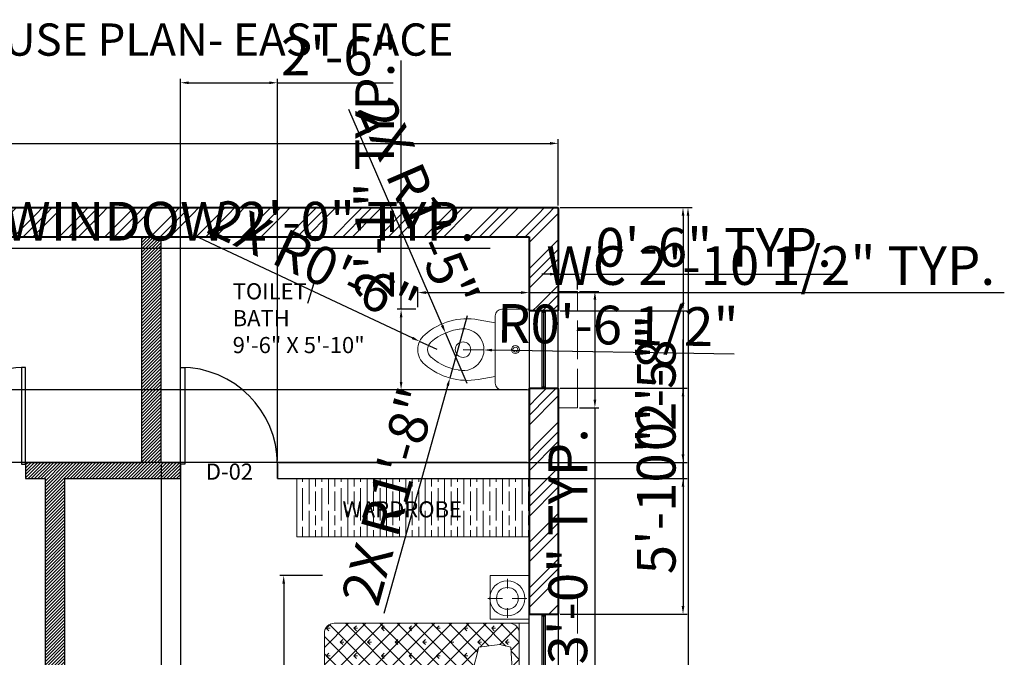
# Model space of a CAD drawing. Units: inches. Extents: x 2386 to 3029, y 792 to 1465.
# Tile 12 of 12: x 2724 to 3029, y 1249 to 1446. Entities that reach past the tile are written whole.
import ezdxf

# ---------------------------------------------------------------- set-up
doc = ezdxf.new("R2010")
doc.units = ezdxf.units.IN
doc.linetypes.add('ACAD_ISO02W100', pattern=[15, 12, -3])
for name, color, linetype, lineweight in [('A-AREA-IDEN', 4, 'Continuous', 25), ('A-DIMS', 1, 'Continuous', 18), ('A-DOOR', 2, 'Continuous', 25), ('A-FLOR-CASE', 6, 'Continuous', 18), ('A-FLOR-CASE-PATT', 9, 'Continuous', 13), ('A-FLOR-FIXT', 9, 'Continuous', 18), ('A-FURN', 6, 'Continuous', 18), ('A-TEXT', 4, 'Continuous', 25), ('A-WALL-EXT', 7, 'Continuous', 40), ('A-WALL-INT', 9, 'Continuous', 30), ('A-WALL-PATT', 9, 'Continuous', 13), ('A-WINDOW', 4, 'Continuous', 25), ('A-WINDOW-OVHD', 4, 'ACAD_ISO02W100', 18)]:
    doc.layers.add(name, color=color, linetype=linetype, lineweight=lineweight)
doc.styles.get("Standard").update_dxf_attribs({"font": 'arial.ttf'})
doc.dimstyles.new('ISO-25', dxfattribs={"dimtxt": 12, "dimasz": 2.5, "dimexe": 1.25, "dimexo": 0.625, "dimtad": 1, "dimlunit": 4, "dimtxsty": 'Standard', "dimcen": 2.5, "dimadec": 0, "dimazin": 0, "dimtfac": 1, "dimtmove": 0, "dimatfit": 3, "dimfxl": 1, "dimarcsym": 0})

# ---------------------------------------------------------------- blocks, each defined once
blk = doc.blocks.new('*X5')
at = {"color": 0}
for p, q in [((0, 0), (0, 0)), ((-566, 0), (-566, 0)), ((-566, 0), (-566, 0)), ((-283, 0), (-283, 0)), ((-283, 0), (-283, 0)), ((283, 0), (283, 0)), ((566, 0), (566, 0)), ((-707, -141), (-734, -115)), ((-707, -141), (-707, -104)), ((-707, -141), (-681, -115)), ((-156, -126), (-168, -115)), ((-141, -141), (-142, -140)), ((-141, -141), (-141, -104)), ((-141, -141), (-115, -115)), ((120, -120), (115, -115)), ((699, -134), (681, -115)), ((707, -135), (707, -104)), ((710, -139), (734, -115)), ((-849, -283), (-875, -256)), ((-849, -283), (-849, -245)), ((-849, -283), (-822, -256)), ((0, -283), (-27, -256)), ((0, -283), (0, -245)), ((0, -283), (27, -256)), ((849, -283), (822, -256)), ((849, -283), (849, -245)), ((849, -283), (875, -256)), ((-707, -424), (-734, -398)), ((-707, -424), (-707, -387)), ((-707, -424), (-681, -398)), ((-116, -399), (-115, -398)), ((707, -424), (707, -387)), ((707, -424), (734, -398)), ((707, -424), (703, -420)), ((-849, -566), (-875, -539)), ((-849, -566), (-849, -528)), ((-849, -566), (-822, -539)), ((-566, -566), (-592, -539)), ((-566, -566), (-566, -528)), ((-566, -566), (-539, -539)), ((-283, -566), (-309, -539)), ((-283, -566), (-283, -528)), ((-283, -566), (-256, -539)), ((0, -566), (-27, -539)), ((0, -566), (0, -528)), ((0, -566), (27, -539)), ((283, -566), (256, -539)), ((283, -566), (283, -528)), ((283, -566), (309, -539)), ((566, -566), (539, -539)), ((566, -566), (566, -528)), ((566, -566), (592, -539)), ((849, -566), (822, -539)), ((849, -566), (849, -528)), ((849, -566), (875, -539)), ((-707, -707), (-734, -681)), ((-707, -707), (-707, -670)), ((-707, -707), (-681, -681)), ((-424, -707), (-451, -681)), ((-424, -707), (-424, -670)), ((-424, -707), (-398, -681)), ((-141, -707), (-168, -681)), ((-141, -707), (-141, -670)), ((-141, -707), (-115, -681)), ((141, -707), (115, -681)), ((141, -707), (141, -670)), ((141, -707), (168, -681)), ((424, -707), (398, -681)), ((424, -707), (424, -670)), ((424, -707), (451, -681)), ((707, -707), (681, -681)), ((707, -707), (707, -670)), ((707, -707), (734, -681)), ((-849, -849), (-875, -822)), ((-849, -849), (-849, -811)), ((-849, -849), (-822, -822)), ((-566, -849), (-592, -822)), ((-566, -849), (-566, -811)), ((-566, -849), (-539, -822)), ((-283, -849), (-309, -822)), ((-283, -849), (-283, -811)), ((-283, -849), (-256, -822)), ((0, -849), (-27, -822)), ((0, -849), (0, -811)), ((0, -849), (27, -822)), ((283, -849), (256, -822)), ((283, -849), (283, -811)), ((283, -849), (309, -822)), ((566, -849), (539, -822)), ((566, -849), (566, -811)), ((566, -849), (592, -822)), ((849, -849), (822, -822)), ((849, -849), (849, -811)), ((849, -849), (875, -822)), ((-707, -990), (-734, -963)), ((-707, -990), (-707, -952)), ((-707, -990), (-681, -963)), ((-424, -990), (-451, -963)), ((-424, -990), (-424, -952)), ((-424, -990), (-398, -963)), ((-141, -990), (-168, -963)), ((-141, -990), (-141, -952)), ((-141, -990), (-115, -963)), ((141, -990), (115, -963)), ((141, -990), (141, -952)), ((141, -990), (168, -963)), ((424, -990), (398, -963)), ((424, -990), (424, -952)), ((424, -990), (451, -963)), ((707, -990), (681, -963)), ((707, -990), (707, -952)), ((707, -990), (734, -963)), ((-849, -1131), (-875, -1105)), ((-849, -1131), (-849, -1094)), ((-849, -1131), (-822, -1105)), ((-566, -1131), (-592, -1105)), ((-566, -1131), (-566, -1094)), ((-566, -1131), (-539, -1105)), ((-283, -1131), (-309, -1105)), ((-283, -1131), (-283, -1094)), ((-283, -1131), (-256, -1105)), ((0, -1131), (-27, -1105)), ((0, -1131), (0, -1094)), ((0, -1131), (27, -1105)), ((283, -1131), (256, -1105)), ((283, -1131), (283, -1094)), ((283, -1131), (309, -1105)), ((566, -1131), (539, -1105)), ((566, -1131), (566, -1094)), ((566, -1131), (592, -1105)), ((849, -1131), (822, -1105)), ((849, -1131), (849, -1094)), ((849, -1131), (875, -1105)), ((-707, -1273), (-734, -1246)), ((-707, -1273), (-707, -1235)), ((-707, -1273), (-681, -1246)), ((-424, -1273), (-451, -1246)), ((-424, -1273), (-424, -1235)), ((-424, -1273), (-398, -1246)), ((-141, -1273), (-168, -1246)), ((-141, -1273), (-141, -1235)), ((-141, -1273), (-115, -1246)), ((141, -1273), (115, -1246)), ((141, -1273), (141, -1235)), ((141, -1273), (168, -1246)), ((424, -1273), (398, -1246)), ((424, -1273), (424, -1235)), ((424, -1273), (451, -1246)), ((707, -1273), (681, -1246)), ((707, -1273), (707, -1235)), ((707, -1273), (734, -1246)), ((-849, -1414), (-875, -1388)), ((-849, -1414), (-849, -1377)), ((-849, -1414), (-822, -1388)), ((-566, -1414), (-592, -1388)), ((-566, -1414), (-566, -1377)), ((-566, -1414), (-539, -1388)), ((-283, -1414), (-309, -1388)), ((-283, -1414), (-283, -1377)), ((-283, -1414), (-256, -1388)), ((0, -1414), (-27, -1388)), ((0, -1414), (0, -1377)), ((0, -1414), (27, -1388)), ((283, -1414), (256, -1388)), ((283, -1414), (283, -1377)), ((283, -1414), (309, -1388)), ((566, -1414), (539, -1388)), ((566, -1414), (566, -1377)), ((566, -1414), (592, -1388)), ((849, -1414), (822, -1388)), ((849, -1414), (849, -1377)), ((849, -1414), (875, -1388)), ((-707, -1556), (-734, -1529)), ((-707, -1556), (-707, -1518)), ((-707, -1556), (-681, -1529)), ((-424, -1556), (-451, -1529)), ((-424, -1556), (-424, -1518)), ((-424, -1556), (-398, -1529)), ((-141, -1556), (-168, -1529)), ((-141, -1556), (-141, -1518)), ((-141, -1556), (-115, -1529)), ((141, -1556), (115, -1529)), ((141, -1556), (141, -1518)), ((141, -1556), (168, -1529)), ((424, -1556), (398, -1529)), ((424, -1556), (424, -1518)), ((424, -1556), (451, -1529)), ((707, -1556), (681, -1529)), ((707, -1556), (707, -1518)), ((707, -1556), (734, -1529)), ((-849, -1697), (-875, -1671)), ((-849, -1697), (-849, -1660)), ((-849, -1697), (-822, -1671)), ((-566, -1697), (-592, -1671)), ((-566, -1697), (-566, -1660)), ((-566, -1697), (-539, -1671)), ((-283, -1697), (-309, -1671)), ((-283, -1697), (-283, -1660)), ((-283, -1697), (-256, -1671)), ((0, -1697), (-27, -1671)), ((0, -1697), (0, -1660)), ((0, -1697), (27, -1671)), ((283, -1697), (256, -1671)), ((283, -1697), (283, -1660)), ((283, -1697), (309, -1671)), ((566, -1697), (539, -1671)), ((566, -1697), (566, -1660)), ((566, -1697), (592, -1671)), ((849, -1697), (822, -1671)), ((849, -1697), (849, -1660)), ((849, -1697), (875, -1671)), ((-707, -1838), (-734, -1812)), ((-707, -1838), (-707, -1801)), ((-707, -1838), (-681, -1812)), ((-424, -1838), (-451, -1812)), ((-424, -1838), (-424, -1801)), ((-424, -1838), (-398, -1812)), ((-141, -1838), (-168, -1812)), ((-141, -1838), (-141, -1801)), ((-141, -1838), (-115, -1812)), ((141, -1838), (115, -1812)), ((141, -1838), (141, -1801)), ((141, -1838), (168, -1812)), ((424, -1838), (398, -1812)), ((424, -1838), (424, -1801)), ((424, -1838), (451, -1812)), ((707, -1838), (681, -1812)), ((707, -1838), (707, -1801)), ((707, -1838), (734, -1812)), ((-849, -1980), (-875, -1953)), ((-849, -1980), (-849, -1942)), ((-849, -1980), (-822, -1953)), ((-566, -1980), (-592, -1953)), ((-566, -1980), (-566, -1942)), ((-566, -1980), (-539, -1953)), ((-283, -1980), (-309, -1953)), ((-283, -1980), (-283, -1942)), ((-283, -1980), (-256, -1953)), ((0, -1980), (-27, -1953)), ((0, -1980), (0, -1942)), ((0, -1980), (27, -1953)), ((283, -1980), (256, -1953)), ((283, -1980), (283, -1942)), ((283, -1980), (309, -1953)), ((566, -1980), (539, -1953)), ((566, -1980), (566, -1942)), ((566, -1980), (592, -1953))]:
    blk.add_line(p, q, dxfattribs=at)
blk = doc.blocks.new('*X4')
at = {"color": 0}
for p, q in [((-900, -193), (-707, 0)), ((-623, -84), (-707, 0)), ((-614, -83), (-530, 0)), ((-457, -74), (-530, 0)), ((-425, -72), (-354, 0)), ((-245, -108), (-354, 0)), ((-278, -101), (-177, 0)), ((103, -280), (-177, 0)), ((-142, -142), (0, 0)), ((-117, -294), (177, 0)), ((120, -120), (0, 0)), ((241, -64), (177, 0)), ((292, -61), (354, 0)), ((426, -72), (354, 0)), ((452, -78), (530, 0)), ((654, -123), (530, 0)), ((596, -111), (707, 0)), ((900, -193), (707, 0)), ((-683, -201), (-862, -22)), ((708, -175), (862, -22)), ((-900, -370), (-667, -137)), ((-656, -405), (-900, -161)), ((703, -358), (900, -161)), ((900, -370), (708, -178)), ((-900, -1254), (101, -252)), ((900, -1254), (-128, -225)), ((-900, -546), (-668, -314)), ((735, -1973), (-900, -337)), ((-763, -2000), (900, -337)), ((900, -546), (703, -349)), ((-900, -1430), (112, -418)), ((-900, -723), (-605, -429)), ((-900, -900), (-465, -465)), ((-900, -1077), (-293, -470)), ((-900, -1607), (231, -476)), ((-900, -1784), (394, -489)), ((-888, -1948), (586, -475)), ((801, -1862), (-641, -419)), ((900, -1784), (-404, -480)), ((900, -1607), (-243, -465)), ((900, -1430), (-116, -415)), ((900, -1077), (317, -494)), ((900, -900), (483, -483)), ((900, -723), (647, -470)), ((586, -2000), (-900, -514)), ((-586, -2000), (900, -514)), ((409, -2000), (-900, -691)), ((-409, -2000), (900, -691)), ((232, -2000), (-900, -868)), ((-232, -2000), (900, -868)), ((55, -2000), (-900, -1045)), ((-55, -2000), (900, -1045)), ((-121, -2000), (-900, -1221)), ((121, -2000), (900, -1221)), ((-298, -2000), (-900, -1398)), ((298, -2000), (900, -1398)), ((-475, -2000), (-900, -1575)), ((475, -2000), (900, -1575)), ((-652, -2000), (-900, -1752)), ((790, -1861), (900, -1752)), ((652, -2000), (761, -1890)), ((-835, -1994), (-894, -1935))]:
    blk.add_line(p, q, dxfattribs=at)
blk = doc.blocks.new('A$C190D2546')
at = {"layer": 'A-FURN'}
for p, q in [((285, 1928), (285, 2078)), ((541, 2100), (2341, 2100)), ((541, 1881), (541, 2100)), ((2341, 1881), (2341, 2100)), ((2596, 1929), (2596, 2079)), ((2341, 2000), (541, 2000)), ((185, 1878), (85, 1878)), ((285, 1828), (285, 1678)), ((385, 1878), (485, 1878)), ((2496, 1879), (2396, 1879)), ((2596, 1829), (2596, 1679)), ((2696, 1879), (2796, 1879))]:
    blk.add_line(p, q, dxfattribs=at)
for points in [[(500, 2101), (500, 1701), (50, 1701), (50, 2101)], [(2382, 2101), (2382, 1701), (2832, 1701), (2832, 2101)], [(787, 1584), (758, 1799), (787, 1914), (1016, 1928), (1296, 1871), (1325, 1699), (1325, 1548), (1038, 1519)], [(1555, 1548), (1541, 1771), (1569, 1928), (1799, 1943), (2151, 1864), (2144, 1685), (2144, 1534), (1763, 1505)]]:
    blk.add_lwpolyline(points, close=True, dxfattribs=at)
blk.add_lwpolyline([(641, 2000), (2241, 2000, -0.414214), (2341, 1900), (2341, 100, -0.414214), (2241, 0), (641, 0, -0.414214), (541, 100), (541, 1900, -0.414214)], format="xyb", close=True, dxfattribs=at)
for centre, radius in [((285, 1878), 180), ((2596, 1879), 180), ((285, 1878), 112), ((2596, 1879), 112)]:
    blk.add_circle(centre, radius, dxfattribs=at)
for centre, start, end in [((2091, 100), 296.5651, 26.5651), ((2241, 250), 243.4349, 333.4349)]:
    blk.add_arc(centre, 112, start, end, dxfattribs=at)
for name in ['*X4', '*X5']:
    blk.add_blockref(name, (1441, 2000), dxfattribs=at)
blk = doc.blocks.new('*U3')
for p, q in [((0, 0), (0, -6)), ((-40, 0), (-40, -6))]:
    blk.add_line(p, q)
blk.add_lwpolyline([(0, 0), (0, 40), (-1.75, 40), (-1.75, 0)], close=True)
blk.add_arc((0, 0), 40, 90, 180)
blk = doc.blocks.new('*U16')
for p, q in [((0, 0), (0, -6)), ((40, 0), (40, -6))]:
    blk.add_line(p, q)
blk.add_lwpolyline([(0, 0), (0, 40), (1.75, 40), (1.75, 0)], close=True)
blk.add_arc((0, 0), 40, 0, 90)
blk = doc.blocks.new('*D21')
at = {"layer": 'A-DIMS', "color": 0, "lineweight": -2, "transparency": 16777216}
for p, q in [((2471.19, 1388.57), (2471.19, 1409.12)), ((2473.69, 1407.87), (2888.69, 1407.87)), ((2891.19, 1388.57), (2891.19, 1409.12))]:
    blk.add_line(p, q, dxfattribs=at)
at = {"layer": 'A-DIMS', "color": 0, "transparency": 16777216}
for points in [[(2473.69, 1408.28), (2473.69, 1407.45), (2471.19, 1407.87)], [(2888.69, 1408.28), (2888.69, 1407.45), (2891.19, 1407.87)]]:
    blk.add_solid(points, dxfattribs=at)
at = {"layer": 'Defpoints', "color": 0, "transparency": 16777216}
for p in [(2891.19, 1407.87), (2471.19, 1387.95), (2891.19, 1387.95)]:
    blk.add_point(p, dxfattribs=at)
at = {"layer": 'A-DIMS', "color": 0, "transparency": 16777216, "insert": (2681.19, 1414.62), "char_height": 12, "attachment_point": 5}
blk.add_mtext("35'", dxfattribs=at)
blk = doc.blocks.new('*D22')
at = {"layer": 'A-DIMS', "color": 0, "lineweight": -2, "transparency": 16777216}
for p, q in [((2891.82, 1387.95), (2932.69, 1387.95)), ((2931.44, 1385.45), (2931.44, 850.45)), ((2891.82, 847.95), (2932.69, 847.95))]:
    blk.add_line(p, q, dxfattribs=at)
at = {"layer": 'A-DIMS', "color": 0, "transparency": 16777216}
for points in [[(2931.02, 1385.45), (2931.85, 1385.45), (2931.44, 1387.95)], [(2931.02, 850.45), (2931.85, 850.45), (2931.44, 847.95)]]:
    blk.add_solid(points, dxfattribs=at)
at = {"layer": 'Defpoints', "color": 0, "transparency": 16777216}
for p in [(2891.19, 1387.95), (2891.19, 847.95), (2931.44, 847.95)]:
    blk.add_point(p, dxfattribs=at)
at = {"layer": 'A-DIMS', "color": 0, "transparency": 16777216, "insert": (2924.71, 1117.95), "char_height": 12, "attachment_point": 5, "rotation": 90}
blk.add_mtext("45'", dxfattribs=at)
blk = doc.blocks.new('WC-FLOOR-MOUNT')
for p, q in [((34.48, 25), (26.06, 25)), ((18.75, 21.75), (23.99, 20.83)), ((24, 22.94), (24, 2.06)), ((18.75, 3.25), (23.99, 4.16)), ((34.48, 0), (26.06, 0))]:
    blk.add_line(p, q)
for centre, radius in [((14.02, 12.49), 2.41), ((30.25, 12.5), 1.25), ((30.25, 12.5), 0.75)]:
    blk.add_circle(centre, radius)
for centre, radius, start, end in [((26.06, 22.94), 2.06, 90, 180), ((15.32, 2.04), 20, 80.1061, 131.065), ((15.32, 2.04), 17, 95.686, 131.065), ((14.02, 12.49), 6.48, 257.3713, 100.6839), ((6, 12.5), 6, 129.5742, 180), ((6, 12.5), 6, 180, 230.4258), ((6, 12.5), 3, 129.5742, 180), ((6, 12.5), 3, 180, 230.4258), ((15.32, 22.95), 17, 228.935, 265.0633), ((15.32, 22.95), 20, 228.935, 279.8939), ((26.06, 2.06), 2.06, 180, 270)]:
    blk.add_arc(centre, radius, start, end)
blk = doc.blocks.new('WINDOW-60IN')
for p, q in [((0, 0), (0, 60)), ((0, 60), (9, 60)), ((4, 60), (4, 0)), ((4, 59.5), (5, 59.5)), ((4.5, 59.5), (4.5, 0.5)), ((5, 60), (5, 0)), ((9, 60), (9, 0)), ((0, 0), (9, 0)), ((5, 0.5), (4, 0.5))]:
    blk.add_line(p, q)
blk = doc.blocks.new('WINDOW-HOOD-60IN')
for p, q in [((0, 72), (6, 72)), ((6, 72), (6, 0)), ((0, 0), (6, 0))]:
    blk.add_line(p, q)
blk = doc.blocks.new('WINDOW-24IN')
for p, q in [((24, 9), (0, 9)), ((0, 0), (0, 9)), ((24, 0), (24, 9)), ((0, 5), (24, 5)), ((0, 4), (24, 4)), ((0.5, 5), (0.5, 4)), ((0.5, 4.5), (23.5, 4.5)), ((23.5, 4), (23.5, 5)), ((0, 0), (24, 0))]:
    blk.add_line(p, q)
blk = doc.blocks.new('WINDOW-HOOD-24IN')
for p, q in [((36, 6), (0, 6)), ((0, 0), (0, 6)), ((36, 0), (36, 6))]:
    blk.add_line(p, q)
blk = doc.blocks.new('*D34')
at = {"layer": 'A-DIMS', "color": 0, "lineweight": -2, "transparency": 16777216}
for p, q in [((2818.13, 1273.95), (2804.91, 1273.95)), ((2806.16, 1271.45), (2806.16, 1192.45)), ((2818.13, 1189.95), (2804.91, 1189.95)), ((2806.16, 1189.95), (2806.16, 1037.2))]:
    blk.add_line(p, q, dxfattribs=at)
at = {"layer": 'A-DIMS', "color": 0, "transparency": 16777216}
for points in [[(2805.74, 1271.45), (2806.57, 1271.45), (2806.16, 1273.95)], [(2805.74, 1192.45), (2806.57, 1192.45), (2806.16, 1189.95)]]:
    blk.add_solid(points, dxfattribs=at)
at = {"layer": 'Defpoints', "color": 0, "transparency": 16777216}
for p in [(2818.76, 1273.95), (2806.16, 1189.95), (2818.76, 1189.95)]:
    blk.add_point(p, dxfattribs=at)
at = {"layer": 'A-DIMS', "color": 0, "transparency": 16777216, "insert": (2799.33, 1112.32), "char_height": 12, "attachment_point": 5, "rotation": 90}
blk.add_mtext('BED SET 7\'-0" TYP.', dxfattribs=at)
blk = doc.blocks.new('*D48')
at = {"layer": 'A-DIMS', "color": 0, "lineweight": -2, "transparency": 16777216}
for p, q in [((2642.19, 1378.32), (2642.19, 1374.1)), ((2666.19, 1378.32), (2666.19, 1374.1)), ((2644.69, 1375.35), (2663.69, 1375.35)), ((2666.19, 1375.35), (2870.13, 1375.35))]:
    blk.add_line(p, q, dxfattribs=at)
at = {"layer": 'A-DIMS', "color": 0, "transparency": 16777216}
for points in [[(2644.69, 1375.76), (2644.69, 1374.93), (2642.19, 1375.35)], [(2663.69, 1375.76), (2663.69, 1374.93), (2666.19, 1375.35)]]:
    blk.add_solid(points, dxfattribs=at)
at = {"layer": 'Defpoints', "color": 0, "transparency": 16777216}
for p in [(2642.19, 1378.95), (2666.19, 1378.95), (2666.19, 1375.35)]:
    blk.add_point(p, dxfattribs=at)
at = {"layer": 'A-DIMS', "color": 0, "transparency": 16777216, "insert": (2769.41, 1382.18), "char_height": 12, "attachment_point": 5}
blk.add_mtext('BATH WINDOW 2\'-0" TYP.', dxfattribs=at)
blk = doc.blocks.new('*D50')
at = {"layer": 'A-DIMS', "color": 0, "lineweight": -2, "transparency": 16777216}
for p, q in [((2897.82, 1361.95), (2903.84, 1361.95)), ((2902.59, 1359.45), (2902.59, 1328.45)), ((2897.82, 1325.95), (2903.84, 1325.95)), ((2902.59, 1325.95), (2902.59, 1145.27))]:
    blk.add_line(p, q, dxfattribs=at)
at = {"layer": 'A-DIMS', "color": 0, "transparency": 16777216}
for points in [[(2902.17, 1359.45), (2903.01, 1359.45), (2902.59, 1361.95)], [(2902.17, 1328.45), (2903.01, 1328.45), (2902.59, 1325.95)]]:
    blk.add_solid(points, dxfattribs=at)
at = {"layer": 'Defpoints', "color": 0, "transparency": 16777216}
for p in [(2897.19, 1361.95), (2897.19, 1325.95), (2902.59, 1325.95)]:
    blk.add_point(p, dxfattribs=at)
at = {"layer": 'A-DIMS', "color": 0, "transparency": 16777216, "insert": (2895.75, 1234.36), "char_height": 12, "attachment_point": 5, "rotation": 90}
blk.add_mtext('BATH HOOD 3\'-0" TYP.', dxfattribs=at)
blk = doc.blocks.new('*D51')
at = {"layer": 'A-DIMS', "color": 0, "lineweight": -2, "transparency": 16777216}
for p, q in [((2888.69, 1367.35), (2886.19, 1367.35)), ((2891.19, 1362.57), (2891.19, 1368.6)), ((2891.19, 1367.35), (2897.19, 1367.35)), ((2897.19, 1362.57), (2897.19, 1368.6)), ((2899.69, 1367.35), (2976.59, 1367.35))]:
    blk.add_line(p, q, dxfattribs=at)
at = {"layer": 'A-DIMS', "color": 0, "transparency": 16777216}
for points in [[(2888.69, 1367.76), (2888.69, 1366.93), (2891.19, 1367.35)], [(2899.69, 1367.76), (2899.69, 1366.93), (2897.19, 1367.35)]]:
    blk.add_solid(points, dxfattribs=at)
at = {"layer": 'Defpoints', "color": 0, "transparency": 16777216}
for p in [(2897.19, 1367.35), (2891.19, 1361.95), (2897.19, 1361.95)]:
    blk.add_point(p, dxfattribs=at)
at = {"layer": 'A-DIMS', "color": 0, "transparency": 16777216, "insert": (2939.39, 1374.1), "char_height": 12, "attachment_point": 5}
blk.add_mtext('0\'-6" TYP.', dxfattribs=at)
blk = doc.blocks.new('*D54')
at = {"layer": 'A-DIMS', "color": 0, "lineweight": -2, "transparency": 16777216}
for p, q in [((2847.71, 1357.07), (2847.71, 1362.87)), ((2850.21, 1361.62), (2879.69, 1361.62)), ((2882.19, 1357.07), (2882.19, 1362.87)), ((2882.19, 1361.62), (3029.45, 1361.62))]:
    blk.add_line(p, q, dxfattribs=at)
at = {"layer": 'A-DIMS', "color": 0, "transparency": 16777216}
for points in [[(2850.21, 1362.04), (2850.21, 1361.2), (2847.71, 1361.62)], [(2879.69, 1362.04), (2879.69, 1361.2), (2882.19, 1361.62)]]:
    blk.add_solid(points, dxfattribs=at)
at = {"layer": 'Defpoints', "color": 0, "transparency": 16777216}
for p in [(2882.19, 1361.62), (2847.71, 1356.45), (2882.19, 1356.45)]:
    blk.add_point(p, dxfattribs=at)
at = {"layer": 'A-DIMS', "color": 0, "transparency": 16777216, "insert": (2957.07, 1368.45), "char_height": 12, "attachment_point": 5}
blk.add_mtext('WC 2\'-10 1/2" TYP.', dxfattribs=at)
blk = doc.blocks.new('*D55')
at = {"layer": 'A-DIMS', "color": 0, "lineweight": -2, "transparency": 16777216}
for p, q in [((2842.53, 1356.45), (2842.53, 1433.55)), ((2847.08, 1356.45), (2841.28, 1356.45)), ((2842.53, 1333.95), (2842.53, 1353.95)), ((2847.08, 1331.45), (2841.28, 1331.45))]:
    blk.add_line(p, q, dxfattribs=at)
at = {"layer": 'A-DIMS', "color": 0, "transparency": 16777216}
for points in [[(2842.12, 1353.95), (2842.95, 1353.95), (2842.53, 1356.45)], [(2842.12, 1333.95), (2842.95, 1333.95), (2842.53, 1331.45)]]:
    blk.add_solid(points, dxfattribs=at)
at = {"layer": 'Defpoints', "color": 0, "transparency": 16777216}
for p in [(2842.53, 1356.45), (2847.71, 1356.45), (2847.71, 1331.45)]:
    blk.add_point(p, dxfattribs=at)
at = {"layer": 'A-DIMS', "color": 0, "transparency": 16777216, "insert": (2835.88, 1396.25), "char_height": 12, "attachment_point": 5, "rotation": 90}
blk.add_mtext('2\'-1" TYP.', dxfattribs=at)
blk = doc.blocks.new('*D58')
at = {"layer": 'A-DIMS', "color": 0, "lineweight": -2, "transparency": 16777216}
for p, q in [((2774.19, 1309.57), (2774.19, 1427.9)), ((2804.19, 1309.57), (2804.19, 1427.9)), ((2776.69, 1426.65), (2801.69, 1426.65)), ((2804.19, 1426.65), (2840.04, 1426.65))]:
    blk.add_line(p, q, dxfattribs=at)
at = {"layer": 'A-DIMS', "color": 0, "transparency": 16777216}
for points in [[(2776.69, 1427.06), (2776.69, 1426.23), (2774.19, 1426.65)], [(2801.69, 1427.06), (2801.69, 1426.23), (2804.19, 1426.65)]]:
    blk.add_solid(points, dxfattribs=at)
at = {"layer": 'Defpoints', "color": 0, "transparency": 16777216}
for p in [(2804.19, 1426.65), (2774.19, 1308.95), (2804.19, 1308.95)]:
    blk.add_point(p, dxfattribs=at)
at = {"layer": 'A-DIMS', "color": 0, "transparency": 16777216, "insert": (2823.37, 1433.4), "char_height": 12, "attachment_point": 5}
blk.add_mtext('2\'-6"', dxfattribs=at)
blk = doc.blocks.new('*D59')
at = {"layer": 'A-DIMS', "color": 0, "lineweight": -2, "transparency": 16777216}
for p, q in [((2768.19, 1308.32), (2768.19, 808)), ((2774.19, 1308.32), (2774.19, 808)), ((2765.69, 809.25), (2763.19, 809.25)), ((2768.19, 809.25), (2774.19, 809.25)), ((2776.69, 809.25), (2812.34, 809.25))]:
    blk.add_line(p, q, dxfattribs=at)
at = {"layer": 'A-DIMS', "color": 0, "transparency": 16777216}
for points in [[(2765.69, 809.66), (2765.69, 808.83), (2768.19, 809.25)], [(2776.69, 809.66), (2776.69, 808.83), (2774.19, 809.25)]]:
    blk.add_solid(points, dxfattribs=at)
at = {"layer": 'Defpoints', "color": 0, "transparency": 16777216}
for p in [(2768.19, 1308.95), (2774.19, 1308.95), (2774.19, 809.25)]:
    blk.add_point(p, dxfattribs=at)
at = {"layer": 'A-DIMS', "color": 0, "transparency": 16777216, "insert": (2795.76, 816), "char_height": 12, "attachment_point": 5}
blk.add_mtext('0\'-6"', dxfattribs=at)
blk = doc.blocks.new('*D67')
at = {"layer": 'A-DIMS', "color": 0, "lineweight": -2, "transparency": 16777216}
for p, q in [((2891.82, 1387.95), (2931.14, 1387.95)), ((2929.89, 1385.45), (2929.89, 1358.45)), ((2891.82, 1355.95), (2931.14, 1355.95)), ((2929.89, 1355.95), (2929.89, 1320.09))]:
    blk.add_line(p, q, dxfattribs=at)
at = {"layer": 'A-DIMS', "color": 0, "transparency": 16777216}
for points in [[(2929.47, 1385.45), (2930.31, 1385.45), (2929.89, 1387.95)], [(2929.47, 1358.45), (2930.31, 1358.45), (2929.89, 1355.95)]]:
    blk.add_solid(points, dxfattribs=at)
at = {"layer": 'Defpoints', "color": 0, "transparency": 16777216}
for p in [(2891.19, 1387.95), (2891.19, 1355.95), (2929.89, 1355.95)]:
    blk.add_point(p, dxfattribs=at)
at = {"layer": 'A-DIMS', "color": 0, "transparency": 16777216, "insert": (2923.14, 1336.77), "char_height": 12, "attachment_point": 5, "rotation": 90}
blk.add_mtext('2\'-8"', dxfattribs=at)
blk = doc.blocks.new('*D68')
at = {"layer": 'A-DIMS', "color": 0, "lineweight": -2, "transparency": 16777216}
for p, q in [((2891.82, 1331.95), (2931.14, 1331.95)), ((2929.89, 1329.45), (2929.89, 1264.45)), ((2891.82, 1261.95), (2931.14, 1261.95))]:
    blk.add_line(p, q, dxfattribs=at)
at = {"layer": 'A-DIMS', "color": 0, "transparency": 16777216}
for points in [[(2929.47, 1329.45), (2930.31, 1329.45), (2929.89, 1331.95)], [(2929.47, 1264.45), (2930.31, 1264.45), (2929.89, 1261.95)]]:
    blk.add_solid(points, dxfattribs=at)
at = {"layer": 'Defpoints', "color": 0, "transparency": 16777216}
for p in [(2891.19, 1331.95), (2891.19, 1261.95), (2929.89, 1261.95)]:
    blk.add_point(p, dxfattribs=at)
at = {"layer": 'A-DIMS', "color": 0, "transparency": 16777216, "insert": (2923.14, 1296.95), "char_height": 12, "attachment_point": 5, "rotation": 90}
blk.add_mtext('5\'-10"', dxfattribs=at)
blk = doc.blocks.new('*D89')
at = {"layer": 'A-DIMS', "color": 0, "lineweight": -2, "transparency": 16777216}
for p, q in [((2432.49, 1331.45), (2432.49, 1403.25)), ((2881.57, 1331.45), (2431.24, 1331.45)), ((2432.49, 1311.45), (2432.49, 1328.95)), ((2881.57, 1308.95), (2431.24, 1308.95))]:
    blk.add_line(p, q, dxfattribs=at)
at = {"layer": 'A-DIMS', "color": 0, "transparency": 16777216}
for points in [[(2432.07, 1328.95), (2432.91, 1328.95), (2432.49, 1331.45)], [(2432.07, 1311.45), (2432.91, 1311.45), (2432.49, 1308.95)]]:
    blk.add_solid(points, dxfattribs=at)
at = {"layer": 'Defpoints', "color": 0, "transparency": 16777216}
for p in [(2432.49, 1331.45), (2882.19, 1331.45), (2882.19, 1308.95)]:
    blk.add_point(p, dxfattribs=at)
at = {"layer": 'A-DIMS', "color": 0, "transparency": 16777216, "insert": (2425.66, 1368.6), "char_height": 12, "attachment_point": 5, "rotation": 90}
blk.add_mtext('1\'-10 1/2"', dxfattribs=at)
blk = doc.blocks.new('*D90')
at = {"layer": 'A-DIMS', "color": 0, "lineweight": -2, "transparency": 16777216}
for p, q in [((2929.89, 1311.45), (2929.89, 1347.1)), ((2804.82, 1308.95), (2931.14, 1308.95)), ((2929.89, 1303.95), (2929.89, 1308.95)), ((2804.82, 1303.95), (2931.14, 1303.95)), ((2929.89, 1301.45), (2929.89, 1298.95))]:
    blk.add_line(p, q, dxfattribs=at)
at = {"layer": 'A-DIMS', "color": 0, "transparency": 16777216}
for points in [[(2929.47, 1311.45), (2930.31, 1311.45), (2929.89, 1308.95)], [(2929.47, 1301.45), (2930.31, 1301.45), (2929.89, 1303.95)]]:
    blk.add_solid(points, dxfattribs=at)
at = {"layer": 'Defpoints', "color": 0, "transparency": 16777216}
for p in [(2804.19, 1308.95), (2929.89, 1308.95), (2804.19, 1303.95)]:
    blk.add_point(p, dxfattribs=at)
at = {"layer": 'A-DIMS', "color": 0, "transparency": 16777216, "insert": (2923.14, 1330.52), "char_height": 12, "attachment_point": 5, "rotation": 90}
blk.add_mtext('0\'-5"', dxfattribs=at)
blk = doc.blocks.new('*D105')
at = {"layer": 'A-DIMS', "color": 0, "lineweight": -2, "transparency": 16777216}
for p, q in [((2863.02, 1354.4), (2857.65, 1335.14)), ((2837.33, 1262.3), (2856.98, 1332.73))]:
    blk.add_line(p, q, dxfattribs=at)
at = {"layer": 'A-DIMS', "color": 0, "transparency": 16777216}
blk.add_solid([(2856.57, 1332.84), (2857.38, 1332.62), (2857.65, 1335.14)], dxfattribs=at)
at = {"layer": 'Defpoints', "color": 0, "transparency": 16777216}
for p in [(2863.02, 1354.4), (2857.65, 1335.14)]:
    blk.add_point(p, dxfattribs=at)
at = {"layer": 'A-DIMS', "color": 0, "transparency": 16777216, "insert": (2840.31, 1298.12), "char_height": 12, "attachment_point": 5, "rotation": 74.413}
blk.add_mtext('2X R1\'-8"', dxfattribs=at)
blk = doc.blocks.new('*D106')
at = {"layer": 'A-DIMS', "color": 0, "lineweight": -2, "transparency": 16777216}
for p, q in [((2826.27, 1418.51), (2855.28, 1351.39)), ((2863.02, 1333.49), (2856.28, 1349.1))]:
    blk.add_line(p, q, dxfattribs=at)
at = {"layer": 'A-DIMS', "color": 0, "transparency": 16777216}
blk.add_solid([(2855.67, 1351.56), (2854.9, 1351.23), (2856.28, 1349.1)], dxfattribs=at)
at = {"layer": 'Defpoints', "color": 0, "transparency": 16777216}
for p in [(2856.28, 1349.1), (2863.02, 1333.49)]:
    blk.add_point(p, dxfattribs=at)
at = {"layer": 'A-DIMS', "color": 0, "transparency": 16777216, "insert": (2846.48, 1388.78), "char_height": 12, "attachment_point": 5, "rotation": 293.3763}
blk.add_mtext('2X R1\'-5"', dxfattribs=at)
blk = doc.blocks.new('*D107')
at = {"layer": 'A-DIMS', "color": 0, "lineweight": -2, "transparency": 16777216}
for p, q in [((2861.73, 1343.94), (2868.2, 1343.83)), ((2945.79, 1342.51), (2870.7, 1343.79))]:
    blk.add_line(p, q, dxfattribs=at)
at = {"layer": 'A-DIMS', "color": 0, "transparency": 16777216}
blk.add_solid([(2870.71, 1344.21), (2870.7, 1343.37), (2868.2, 1343.83)], dxfattribs=at)
at = {"layer": 'Defpoints', "color": 0, "transparency": 16777216}
for p in [(2861.73, 1343.94), (2868.2, 1343.83)]:
    blk.add_point(p, dxfattribs=at)
at = {"layer": 'A-DIMS', "color": 0, "transparency": 16777216, "insert": (2909.61, 1349.96), "char_height": 12, "attachment_point": 5, "rotation": 359.0236}
blk.add_mtext('R0\'-6 1/2"', dxfattribs=at)
blk = doc.blocks.new('*D108')
at = {"layer": 'A-DIMS', "color": 0, "lineweight": -2, "transparency": 16777216}
for p, q in [((2779.86, 1378.72), (2846.02, 1347.57)), ((2853.71, 1343.95), (2848.28, 1346.5))]:
    blk.add_line(p, q, dxfattribs=at)
at = {"layer": 'A-DIMS', "color": 0, "transparency": 16777216}
blk.add_solid([(2846.19, 1347.95), (2845.84, 1347.19), (2848.28, 1346.5)], dxfattribs=at)
at = {"layer": 'Defpoints', "color": 0, "transparency": 16777216}
for p in [(2848.28, 1346.5), (2853.71, 1343.95)]:
    blk.add_point(p, dxfattribs=at)
at = {"layer": 'A-DIMS', "color": 0, "transparency": 16777216, "insert": (2814.68, 1369.79), "char_height": 12, "attachment_point": 5, "rotation": 334.7848}
blk.add_mtext('2X R0\'-6"', dxfattribs=at)

msp = doc.modelspace()

# ---------------------------------------------------------------- hatches: boundary and pattern name
at = {"layer": 'A-FLOR-CASE-PATT'}
h = msp.add_hatch(dxfattribs=at)
h.set_pattern_fill('GOST_WOOD', color=256)
h.paths.add_polyline_path([(2882.19, 1303.948), (2810.19, 1303.948), (2810.19, 1285.948), (2882.19, 1285.948)])
h.paths.add_polyline_path([(2624.19, 1378.948), (2600.19, 1378.948), (2600.19, 1306.948), (2624.19, 1306.948)])
h.paths.add_polyline_path([(2823.021, 1289.11), (2866.657, 1289.11), (2866.657, 1299.414), (2823.021, 1299.414)], flags=24)
h.paths.add_polyline_path([(2618.821, 1319.237), (2618.821, 1362.873), (2608.517, 1362.873), (2608.517, 1319.237)], flags=24)
at = {"layer": 'A-WALL-PATT'}
h = msp.add_hatch(dxfattribs=at)
h.set_pattern_fill('GOST_GROUND', color=256)
h.paths.add_polyline_path([(2480.19, 1276.948), (2471.19, 1276.948), (2471.19, 1211.948), (2480.19, 1211.948)])
h.paths.add_polyline_path([(2480.19, 1378.948), (2510.19, 1378.948), (2510.19, 1378.969), (2523.779, 1378.969), (2580.602, 1378.959), (2580.602, 1378.969), (2594.19, 1378.969), (2642.19, 1378.948), (2642.19, 1387.948), (2471.19, 1387.948), (2471.19, 1336.948), (2480.19, 1336.948)])
h.paths.add_polyline_path([(2891.19, 1387.948), (2666.19, 1387.948), (2666.19, 1378.948), (2882.19, 1378.948), (2882.19, 1355.948), (2891.19, 1355.948)])
h.paths.add_polyline_path([(2891.19, 1331.948), (2882.19, 1331.948), (2882.19, 1331.449), (2882.19, 1261.948), (2891.19, 1261.948)])
h.paths.add_polyline_path([(2891.19, 1201.948), (2882.19, 1201.948), (2882.19, 1189.948), (2882.19, 1159.948), (2882.19, 1117.948), (2891.19, 1117.948)])
h.paths.add_polyline_path([(2891.19, 1057.948), (2882.19, 1057.948), (2882.19, 856.948), (2882.19, 847.948), (2891.19, 847.948)])
h.paths.add_polyline_path([(2594.19, 856.948), (2558.19, 856.948), (2558.19, 847.948), (2594.19, 847.948)])
h.paths.add_polyline_path([(2510.19, 856.948), (2480.19, 856.948), (2480.19, 905.448), (2471.19, 905.448), (2471.19, 847.948), (2510.19, 847.948)])
h.paths.add_polyline_path([(2480.19, 1007.948), (2471.19, 1007.948), (2471.19, 953.448), (2480.19, 953.448)])
h.paths.add_polyline_path([(2480.19, 1103.948), (2471.19, 1103.948), (2471.19, 1043.948), (2480.19, 1043.948)])
h = msp.add_hatch(dxfattribs=at)
h.set_pattern_fill('JIS_WOOD', color=256)
h.paths.add_polyline_path([(2624.19, 1229.948), (2624.19, 1145.948), (2618.19, 1145.948), (2618.19, 1140.548), (2618.19, 1139.948), (2630.19, 1139.948), (2630.19, 1240.948), (2624.19, 1240.948), (2624.19, 1234.948), (2480.19, 1234.948), (2480.19, 1229.948)])
h.paths.add_polyline_path([(2582.19, 1139.948), (2582.19, 1145.948), (2480.19, 1145.948), (2480.19, 1139.948)], flags=17)
h.paths.add_polyline_path([(2480.19, 1007.948), (2480.19, 1001.948), (2546.19, 1001.948), (2546.19, 1007.348), (2546.19, 1007.948)])
h.paths.add_polyline_path([(2594.19, 1007.948), (2582.19, 1007.948), (2582.19, 1001.948), (2588.19, 1001.948), (2588.19, 856.948), (2594.19, 856.948), (2594.19, 914.948), (2606.19, 914.948), (2606.19, 920.948), (2594.19, 920.948)])
h.paths.add_polyline_path([(2738.19, 1015.948), (2882.19, 1015.948), (2882.19, 1021.948), (2738.19, 1021.948), (2738.19, 1111.948), (2732.19, 1111.948), (2732.19, 920.948), (2720.19, 920.948), (2720.19, 914.948), (2732.19, 914.948), (2732.19, 856.948), (2738.19, 856.948)])
h.paths.add_polyline_path([(2660.19, 914.948), (2660.19, 920.948), (2648.19, 920.948), (2648.19, 914.948)])
h.paths.add_polyline_path([(2738.19, 1159.948), (2738.19, 1165.948), (2737.59, 1165.948), (2732.19, 1165.948), (2732.19, 1147.948), (2737.59, 1147.948), (2738.19, 1147.948), (2738.19, 1153.948), (2882.19, 1153.948), (2882.19, 1159.948)])
h.paths.add_polyline_path([(2732.19, 1201.948), (2738.19, 1201.948), (2738.19, 1303.948), (2774.19, 1303.948), (2774.19, 1308.948), (2768.19, 1308.948), (2768.19, 1378.948), (2762.19, 1378.948), (2762.19, 1308.948), (2726.19, 1308.948), (2726.19, 1303.948), (2732.19, 1303.948)])
h.paths.add_polyline_path([(2696.19, 1303.948), (2696.19, 1308.948), (2630.19, 1308.948), (2630.19, 1378.948), (2624.19, 1378.948), (2624.19, 1276.948), (2630.19, 1276.948), (2630.19, 1303.948)])

# ---------------------------------------------------------------- linework, layer by layer
at = {"layer": 'A-FLOR-CASE'}
msp.add_lwpolyline([(2810.19, 1303.948), (2810.19, 1285.948), (2882.19, 1285.948)], dxfattribs=at)
at = {"layer": 'A-FLOR-FIXT'}
msp.add_line((2882.19, 1356.446), (2882.19, 1331.449), dxfattribs=at)
at = {"layer": 'A-WALL-EXT'}
for p, q in [((2666.19, 1387.948), (2891.19, 1387.948)), ((2891.19, 1387.948), (2891.19, 1355.948)), ((2666.19, 1378.948), (2882.19, 1378.948)), ((2882.19, 1378.948), (2882.19, 1355.948)), ((2891.19, 1355.948), (2882.19, 1355.948)), ((2882.19, 1331.948), (2882.19, 1261.948)), ((2882.19, 1331.948), (2891.19, 1331.948)), ((2891.19, 1331.948), (2891.19, 1261.948)), ((2882.19, 1261.948), (2891.19, 1261.948)), ((2882.19, 1261.948), (2891.19, 1261.948))]:
    msp.add_line(p, q, dxfattribs=at)
at = {"layer": 'A-WALL-INT'}
for p, q in [((2762.19, 1308.948), (2762.19, 1378.948)), ((2768.19, 1308.948), (2768.19, 1378.948)), ((2726.19, 1308.948), (2726.19, 1303.948)), ((2726.19, 1308.948), (2762.19, 1308.948)), ((2768.19, 1308.948), (2774.19, 1308.948)), ((2774.19, 1303.948), (2774.19, 1308.948)), ((2804.19, 1303.948), (2804.19, 1308.948)), ((2804.19, 1308.948), (2882.19, 1308.948)), ((2726.19, 1303.948), (2732.19, 1303.948)), ((2732.19, 1303.948), (2732.19, 1201.948)), ((2738.19, 1303.948), (2774.19, 1303.948)), ((2738.19, 1303.948), (2738.19, 1201.948)), ((2804.19, 1303.948), (2882.19, 1303.948))]:
    msp.add_line(p, q, dxfattribs=at)

# ---------------------------------------------------------------- block references
at = {"layer": 'A-DOOR', "xscale": 0.75, "yscale": 0.75, "zscale": 0.75}
for name, p in [('*U3', (2726.19, 1308.448)), ('*U16', (2774.19, 1308.448))]:
    msp.add_blockref(name, p, dxfattribs=at)
at = {"layer": 'A-FLOR-FIXT'}
msp.add_blockref('WC-FLOOR-MOUNT', (2847.705, 1331.449), dxfattribs=at)
at = {"layer": 'A-FURN', "xscale": 0.0301964232523521, "yscale": 0.0301964232523521, "zscale": 0.0301964232523521, "rotation": 270}
msp.add_blockref('A$C190D2546', (2818.757, 1275.458), dxfattribs=at)
at = {"layer": 'A-WINDOW', "rotation": 269.9999999999991}
msp.add_blockref('WINDOW-24IN', (2882.19, 1355.948), dxfattribs=at)
at = {"layer": 'A-WINDOW'}
msp.add_blockref('WINDOW-60IN', (2882.19, 1201.948), dxfattribs=at)
at = {"layer": 'A-WINDOW-OVHD', "rotation": 270.0000000000007}
msp.add_blockref('WINDOW-HOOD-24IN', (2891.19, 1361.948), dxfattribs=at)
at = {"layer": 'A-WINDOW-OVHD'}
msp.add_blockref('WINDOW-HOOD-60IN', (2891.19, 1195.948), dxfattribs=at)

# ---------------------------------------------------------------- texts
at = {"layer": 'A-AREA-IDEN', "char_height": 5, "attachment_point": 1}
for s, insert in [('TOILET/\\PBATH\\P9\'-6" X 5\'-10"', (2790.347, 1364.524)), ('WARDROBE', (2824.356, 1296.929))]:
    msp.add_mtext_dynamic_manual_height_columns(s, width=52.37406, gutter_width=12.5, heights=[0], dxfattribs=dict(at, insert=insert))
at = {"layer": 'A-TEXT', "attachment_point": 1}
for s, width, insert, char_height in [('EASTWOOD RECIDENCE (1575 sq ft) HOUSE PLAN- EAST FACE', 421.50568, (2472.473, 1445.038), 10), ('D-02', 38.22215, (2782.034, 1308.642), 5)]:
    msp.add_mtext_dynamic_manual_height_columns(s, width=width, gutter_width=12.5, heights=[0], dxfattribs=dict(at, insert=insert, char_height=char_height))

# ---------------------------------------------------------------- dimensions: what is measured, and where the dimension line sits
at = {"layer": 'A-DIMS'}
for base, p1, p2, override, picture, middle in [((2804.19, 1426.648), (2774.19, 1308.948), (2804.19, 1308.948), {"dimdec": 1, "dimlfac": 1, "dimrnd": 0, "dimzin": 1, "dimdsep": 46, "dimlunit": 4, "dimfrac": 2}, '*D58', (2823.367, 1433.4)), ((2891.19, 1407.868), (2471.19, 1387.948), (2891.19, 1387.948), {"dimclrd": 0, "dimclre": 0, "dimclrt": 0}, '*D21', (2681.19, 1414.624)), ((2774.19, 809.248), (2768.19, 1308.948), (2774.19, 1308.948), {"dimdec": 1, "dimlfac": 1, "dimrnd": 0, "dimzin": 1, "dimdsep": 46, "dimlunit": 4, "dimfrac": 2}, '*D59', (2795.765, 816))]:
    dim = msp.add_linear_dim(base=base, p1=p1, p2=p2, dimstyle='ISO-25', override=override, dxfattribs=at)
    dim.commit()
    dim.dimension.update_dxf_attribs({"geometry": picture, "text_midpoint": middle})
for base, p1, p2, angle, text, picture, middle in [((2842.532, 1356.446), (2847.705, 1331.449), (2847.705, 1356.446), 90, '<> TYP.', '*D55', (2835.879, 1396.247)), ((2902.59, 1325.948), (2897.19, 1361.948), (2897.19, 1325.948), 270, 'BATH HOOD <> TYP.', '*D50', (2895.752, 1234.358)), ((2806.157, 1189.948), (2818.757, 1273.948), (2818.757, 1189.948), 270, 'BED SET <> TYP.', '*D34', (2799.327, 1112.322))]:
    dim = msp.add_linear_dim(base=base, p1=p1, p2=p2, angle=angle, text=text, dimstyle='ISO-25', override={"dimdec": 1, "dimlfac": 1, "dimrnd": 0, "dimzin": 1, "dimdsep": 46, "dimlunit": 4, "dimfrac": 2}, dxfattribs=at)
    dim.commit()
    dim.dimension.update_dxf_attribs({"geometry": picture, "text_midpoint": middle})
for center, mpoint, picture, middle in [((2863.021, 1333.493), (2856.276, 1349.098), '*D106', (2846.479, 1388.779)), ((2853.705, 1343.948), (2848.277, 1346.504), '*D108', (2814.683, 1369.786)), ((2863.021, 1354.402), (2857.647, 1335.138), '*D105', (2840.312, 1298.123))]:
    dim = msp.add_radius_dim(center=center, mpoint=mpoint, text='2X <>', dimstyle='ISO-25', override={"dimdec": 1, "dimlfac": 1, "dimrnd": 0, "dimzin": 1, "dimdsep": 46, "dimlunit": 4, "dimfrac": 2}, dxfattribs=at)
    dim.commit()
    dim.dimension.update_dxf_attribs({"geometry": picture, "text_midpoint": middle})
for base, p1, p2, text, picture, middle in [((2666.19, 1375.348), (2642.19, 1378.948), (2666.19, 1378.948), 'BATH WINDOW <> TYP.', '*D48', (2769.412, 1382.182)), ((2882.19, 1361.619), (2847.705, 1356.446), (2882.19, 1356.446), 'WC <> TYP.', '*D54', (2957.07, 1368.449)), ((2897.19, 1367.348), (2891.19, 1361.948), (2897.19, 1361.948), '<> TYP.', '*D51', (2939.388, 1374.1))]:
    dim = msp.add_linear_dim(base=base, p1=p1, p2=p2, text=text, dimstyle='ISO-25', override={"dimdec": 1, "dimlfac": 1, "dimrnd": 0, "dimzin": 1, "dimdsep": 46, "dimlunit": 4, "dimfrac": 2}, dxfattribs=at)
    dim.commit()
    dim.dimension.update_dxf_attribs({"geometry": picture, "text_midpoint": middle})
for base, p1, p2, override, picture, middle in [((2432.49, 1331.449), (2882.19, 1308.948), (2882.19, 1331.449), {"dimdec": 1, "dimlfac": 1, "dimrnd": 0, "dimzin": 1, "dimdsep": 46, "dimlunit": 4, "dimfrac": 2}, '*D89', (2425.66, 1368.602)), ((2931.437, 847.948), (2891.19, 1387.948), (2891.19, 847.948), {"dimclrd": 0, "dimclre": 0, "dimclrt": 0}, '*D22', (2924.709, 1117.948)), ((2929.89, 1355.948), (2891.19, 1387.948), (2891.19, 1355.948), {"dimdec": 1, "dimlfac": 1, "dimrnd": 0, "dimzin": 1, "dimdsep": 46, "dimlunit": 4, "dimfrac": 2}, '*D67', (2923.138, 1336.771)), ((2929.89, 1308.948), (2804.19, 1303.948), (2804.19, 1308.948), {"dimdec": 1, "dimlfac": 1, "dimrnd": 0, "dimzin": 1, "dimdsep": 46, "dimlunit": 4, "dimfrac": 2}, '*D90', (2923.138, 1330.522)), ((2929.89, 1261.948), (2891.19, 1331.948), (2891.19, 1261.948), {"dimdec": 1, "dimlfac": 1, "dimrnd": 0, "dimzin": 1, "dimdsep": 46, "dimlunit": 4, "dimfrac": 2}, '*D68', (2923.138, 1296.948))]:
    dim = msp.add_linear_dim(base=base, p1=p1, p2=p2, angle=90, dimstyle='ISO-25', override=override, dxfattribs=at)
    dim.commit()
    dim.dimension.update_dxf_attribs({"geometry": picture, "text_midpoint": middle})
dim = msp.add_radius_dim(center=(2861.726, 1343.942), mpoint=(2868.204, 1343.832), dimstyle='ISO-25', override={"dimdec": 1, "dimlfac": 1, "dimrnd": 0, "dimzin": 1, "dimdsep": 46, "dimlunit": 4, "dimfrac": 2}, dxfattribs=at)
dim.commit()
dim.dimension.update_dxf_attribs({"geometry": '*D107', "text_midpoint": (2909.612, 1349.957)})

doc.saveas('drawing.dxf')
